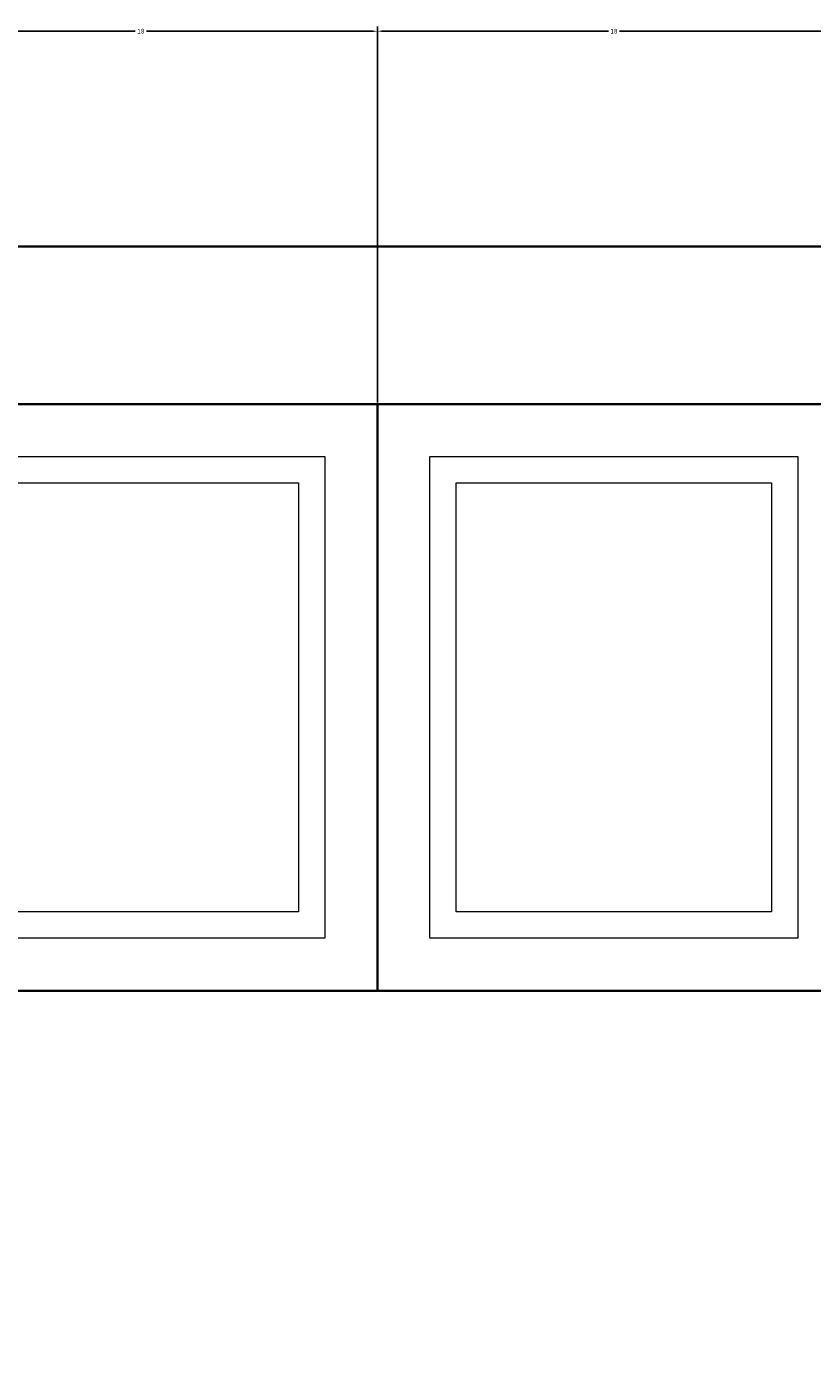
# Model space of a CAD drawing. Units: inches. Extents: x 27 to 200, y -50 to 102.
# Tile 18 of 26: x 89 to 119, y 52 to 102. Entities that reach past the tile are written whole.
import ezdxf

# ---------------------------------------------------------------- set-up
doc = ezdxf.new("R2010")
doc.units = ezdxf.units.IN
doc.header["$MEASUREMENT"] = 0
for name, color, linetype, lineweight in [('A-ANNO-DIMS', 2, 'Continuous', 18), ('A-ELEV', 7, 'Continuous', 35), ('A-FURN', 8, 'Continuous', 18)]:
    doc.layers.add(name, color=color, linetype=linetype, lineweight=lineweight)
doc.styles.get("Standard").update_dxf_attribs({"font": 'arial.ttf'})
doc.dimstyles.get("Standard").update_dxf_attribs({"dimtxt": 0.18, "dimasz": 0.18, "dimexe": 0.18, "dimexo": 0.0625, "dimgap": 0.09, "dimtad": 0, "dimtih": 1, "dimtoh": 1, "dimdec": 4, "dimzin": 0, "dimdsep": 46, "dimtxsty": 'Standard', "dimcen": 0.09, "dimadec": 0, "dimazin": 0, "dimtfac": 1, "dimtdec": 4, "dimtofl": 0, "dimtmove": 0, "dimatfit": 3, "dimfxl": 1, "dimtolj": 1, "dimtzin": 0, "dimarcsym": 0})

# ---------------------------------------------------------------- blocks, each defined once
blk = doc.blocks.new('CAB-DOOR-UPPER')
for p, q in [((0, 0), (0, 18.339)), ((0, 18.339), (14, 18.339)), ((14, 18.339), (14, 0)), ((1, 1), (1, 17.339)), ((1, 17.339), (13, 17.339)), ((13, 17.339), (13, 1)), ((13, 1), (1, 1)), ((14, 0), (0, 0))]:
    blk.add_line(p, q)
blk = doc.blocks.new('*D16')
at = {"layer": 'A-ANNO-DIMS', "color": 0, "lineweight": -2, "transparency": 16777216}
for p, q in [((84.417, 87.989), (84.417, 102.306)), ((102.417, 87.989), (102.417, 102.306)), ((84.597, 102.126), (93.206, 102.126)), ((102.237, 102.126), (93.628, 102.126))]:
    blk.add_line(p, q, dxfattribs=at)
at = {"layer": 'A-ANNO-DIMS', "color": 0, "transparency": 16777216}
for points in [[(84.597, 102.156), (84.597, 102.096), (84.417, 102.126)], [(102.237, 102.156), (102.237, 102.096), (102.417, 102.126)]]:
    blk.add_solid(points, dxfattribs=at)
at = {"layer": 'Defpoints', "color": 0, "transparency": 16777216}
for p in [(102.417, 102.126), (84.417, 87.926), (102.417, 87.926)]:
    blk.add_point(p, dxfattribs=at)
at = {"layer": 'A-ANNO-DIMS', "color": 0, "transparency": 16777216, "insert": (93.417, 102.126), "char_height": 0.18, "attachment_point": 5}
blk.add_mtext('\\A1;18', dxfattribs=at)
blk = doc.blocks.new('*D17')
at = {"layer": 'A-ANNO-DIMS', "color": 0, "lineweight": -2, "transparency": 16777216}
for p, q in [((102.417, 87.989), (102.417, 102.306)), ((120.417, 87.989), (120.417, 102.306)), ((102.597, 102.126), (111.206, 102.126)), ((120.237, 102.126), (111.628, 102.126))]:
    blk.add_line(p, q, dxfattribs=at)
at = {"layer": 'A-ANNO-DIMS', "color": 0, "transparency": 16777216}
for points in [[(102.597, 102.156), (102.597, 102.096), (102.417, 102.126)], [(120.237, 102.156), (120.237, 102.096), (120.417, 102.126)]]:
    blk.add_solid(points, dxfattribs=at)
at = {"layer": 'Defpoints', "color": 0, "transparency": 16777216}
for p in [(120.417, 102.126), (102.417, 87.926), (120.417, 87.926)]:
    blk.add_point(p, dxfattribs=at)
at = {"layer": 'A-ANNO-DIMS', "color": 0, "transparency": 16777216, "insert": (111.417, 102.126), "char_height": 0.18, "attachment_point": 5}
blk.add_mtext('\\A1;18', dxfattribs=at)

msp = doc.modelspace()

# ---------------------------------------------------------------- linework, layer by layer
at = {"layer": 'A-ELEV'}
for p, q in [((191.4169, 93.9264), (35.4169, 93.9264)), ((191.4169, 87.9264), (35.4169, 87.9264)), ((102.4169, 87.9264), (102.4169, 65.5865)), ((84.4169, 65.5865), (120.4169, 65.5865))]:
    msp.add_line(p, q, dxfattribs=at)
msp.add_lwpolyline([(84.4169, 65.5865), (120.4169, 65.5865), (120.4169, 39.8559), (84.4169, 39.8559)], close=True, dxfattribs=at)

# ---------------------------------------------------------------- block references
at = {"layer": 'A-FURN'}
for p in [(86.417, 67.587), (104.417, 67.587)]:
    msp.add_blockref('CAB-DOOR-UPPER', p, dxfattribs=at)

# ---------------------------------------------------------------- dimensions: what is measured, and where the dimension line sits
at = {"layer": 'A-ANNO-DIMS'}
for base, p1, p2, picture, middle in [((102.4169, 102.1264), (84.4169, 87.9264), (102.4169, 87.9264), '*D16', (93.4169, 102.1264)), ((120.4169, 102.1264), (102.4169, 87.9264), (120.4169, 87.9264), '*D17', (111.4169, 102.1264))]:
    dim = msp.add_linear_dim(base=base, p1=p1, p2=p2, dimstyle='Standard', override={"dimdec": 0, "dimlfac": 1, "dimrnd": 0, "dimzin": 0, "dimdsep": 46, "dimlunit": 2}, dxfattribs=at)
    dim.commit()
    dim.dimension.update_dxf_attribs({"geometry": picture, "text_midpoint": middle})

doc.saveas('drawing.dxf')
